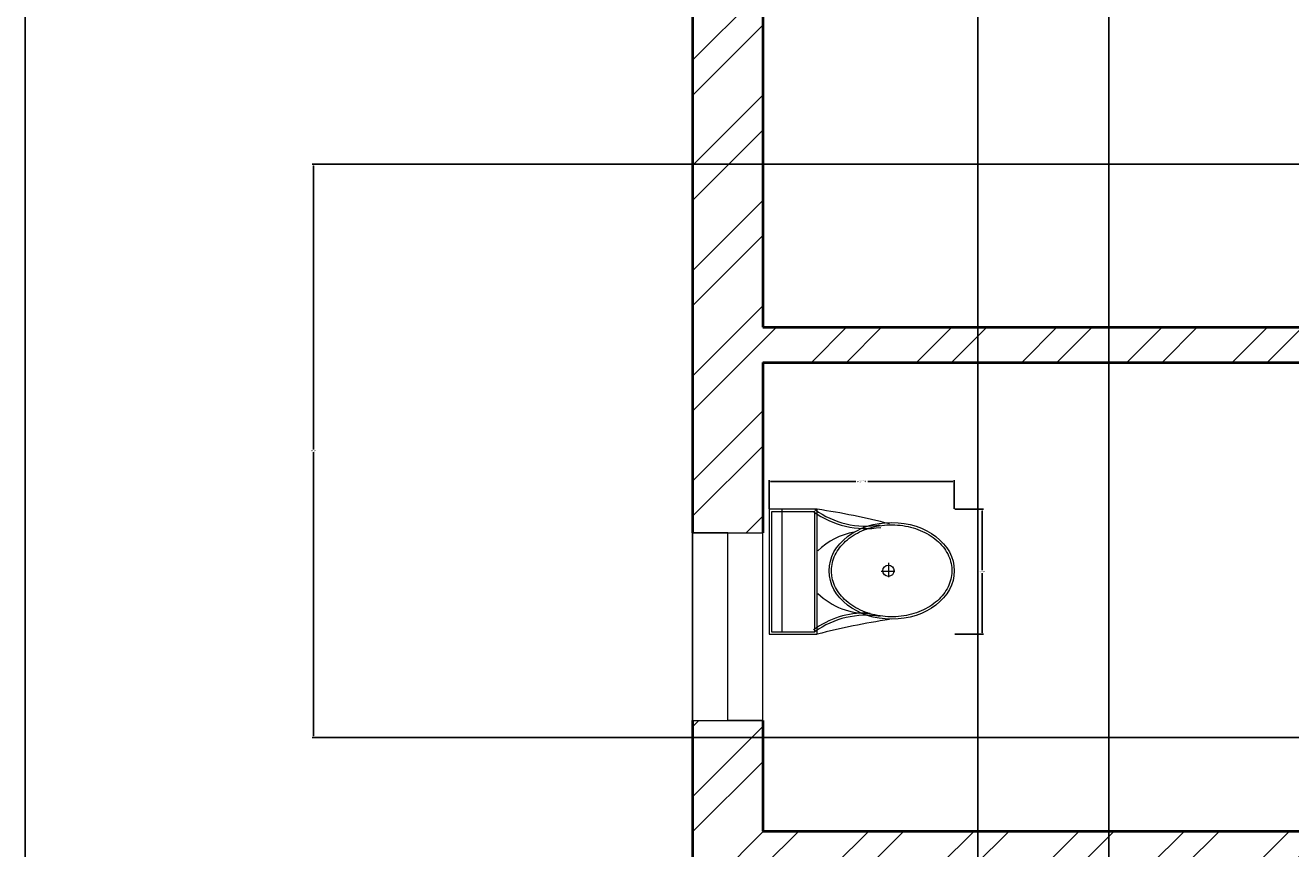
# Model space of a CAD drawing. Units: inches. Extents: x 1601 to 2297, y 1496 to 2631.
# Tile 35 of 57: x 1601 to 1763, y 2286 to 2391. Entities that reach past the tile are written whole.
import ezdxf

# ---------------------------------------------------------------- set-up
doc = ezdxf.new("R2010")
doc.units = ezdxf.units.IN
for name, color, linetype, lineweight in [('A-ANNO-DIMS', 2, 'Continuous', 18), ('A-ANNO-TTLB', 7, 'Continuous', 25), ('A-FLOR-FIXT', 9, 'Continuous', 20), ('A-GLAZ', 161, 'Continuous', 20), ('A-WALL', 7, 'Continuous', 40), ('A-WALL-PATT', 215, 'Continuous', 13)]:
    doc.layers.add(name, color=color, linetype=linetype, lineweight=lineweight)
doc.styles.get("Standard").update_dxf_attribs({"font": 'arial.ttf'})
doc.dimstyles.get("Standard").update_dxf_attribs({"dimtxt": 0.18, "dimasz": 0.18, "dimexe": 0.18, "dimexo": 0.0625, "dimgap": 0.09, "dimtad": 0, "dimtih": 1, "dimtoh": 1, "dimdec": 4, "dimzin": 0, "dimdsep": 46, "dimtxsty": 'Standard', "dimcen": 0.09, "dimadec": 0, "dimazin": 0, "dimtfac": 1, "dimtdec": 4, "dimtofl": 0, "dimtmove": 0, "dimatfit": 3, "dimfxl": 1, "dimtolj": 1, "dimtzin": 0, "dimarcsym": 0})

# ---------------------------------------------------------------- blocks, each defined once
blk = doc.blocks.new('A$C31115884')
for p, q in [((283.1, 497.7), (223.4, 497.7)), ((257.5, 466.4), (257.5, 523.2)), ((0, 200), (0, 0)), ((520, 200), (0, 200)), ((10, 190), (10, 10)), ((510, 190), (10, 190)), ((510, 10), (510, 190)), ((520, 0), (520, 200)), ((510, 54.5), (0, 54.5)), ((10, 10), (510, 10)), ((0, 0), (520, 0))]:
    blk.add_line(p, q)
blk.add_circle((255.6, 496.4), 23.6)
for centre, radius, start, end in [((2777.7, -204.6), 2807, 165.4549, 171.7133), ((3237, 905), 2807, 188.2867, 194.5451), ((-294.5, 403.3), 364.7, 324.2091, 9.3499), ((-294.5, 403.3), 374.7, 324.2091, 9.3499), ((805.8, 403.3), 364.7, 170.6501, 215.7909), ((139.5, 406.2), 293.5, 315.8436, 2.6563), ((805.8, 403.3), 374.7, 179.2036, 215.7909), ((383.6, 406.2), 293.5, 190.2774, 224.1564)]:
    blk.add_arc(centre, radius, start, end)
blk.add_ellipse((256.2, 509.9), major_axis=(0, -260.7), ratio=0.772727)
blk.add_open_spline([(256.2, 259.2), (263.1, 259.2), (270, 259.7), (287.8, 262.3), (298.7, 265.1), (319.9, 273.1), (330.2, 278.4), (350.1, 291.1), (359.7, 298.7), (377.7, 315.9), (386.2, 325.5), (401.7, 346.6), (408.8, 358.1), (421.3, 382.5), (426.8, 395.5), (435.9, 422.4), (439.5, 436.4), (444.8, 465.1), (446.5, 479.7), (447.9, 509.2), (447.6, 524), (445, 553.3), (442.7, 567.8), (436.3, 596), (432.1, 609.7), (421.9, 636), (416, 648.6), (402.5, 672.1), (395, 683), (378.6, 703), (369.8, 712.1), (351.1, 728), (341.3, 734.8), (320.9, 746.2), (310.4, 750.7), (288.9, 757.3), (278, 759.4), (256, 761), (245, 760.6), (223.1, 757.2), (212.3, 754.3), (191.1, 746.1), (180.8, 740.7), (160.9, 727.8), (151.4, 720.1), (133.5, 702.7), (125.1, 693), (109.6, 671.7), (102.6, 660.2), (90.2, 635.7), (84.9, 622.7), (76, 595.6), (72.4, 581.6), (67.2, 552.9), (65.6, 538.2), (64.4, 508.8), (64.8, 494), (67.5, 464.7), (69.9, 450.2), (76.6, 422), (80.8, 408.3), (91.1, 382.2), (97.2, 369.7), (110.8, 346.3), (118.4, 335.4), (134.8, 315.6), (143.7, 306.7), (162.4, 290.9), (172.3, 284.2), (192.8, 273), (203.3, 268.6), (224.8, 262.2), (235.8, 260.2), (249.9, 259.3), (253, 259.2), (256.2, 259.2)], degree=3, knots=[0, 0, 0, 0, 0.110105, 0.110105, 0.285049, 0.285049, 0.459994, 0.459994, 0.634938, 0.634938, 0.809882, 0.809882, 0.984827, 0.984827, 1.159771, 1.159771, 1.334715, 1.334715, 1.50966, 1.50966, 1.684604, 1.684604, 1.859549, 1.859549, 2.034493, 2.034493, 2.209437, 2.209437, 2.384382, 2.384382, 2.559326, 2.559326, 2.73427, 2.73427, 2.909215, 2.909215, 3.084159, 3.084159, 3.259103, 3.259103, 3.434048, 3.434048, 3.608992, 3.608992, 3.783936, 3.783936, 3.958881, 3.958881, 4.133825, 4.133825, 4.30877, 4.30877, 4.483714, 4.483714, 4.658658, 4.658658, 4.833603, 4.833603, 5.008547, 5.008547, 5.183491, 5.183491, 5.358436, 5.358436, 5.53338, 5.53338, 5.708324, 5.708324, 5.883269, 5.883269, 6.058213, 6.058213, 6.233158, 6.233158, 6.283185, 6.283185, 6.283185, 6.283185])
blk = doc.blocks.new('*D10')
at = {"layer": 'A-ANNO-DIMS', "color": 0, "lineweight": -2, "transparency": 16777216}
for p, q in [((1695.85, 2329.09), (1695.85, 2332.76)), ((1696.03, 2332.58), (1706.92, 2332.58)), ((1719.36, 2332.58), (1708.47, 2332.58)), ((1719.54, 2329.09), (1719.54, 2332.76))]:
    blk.add_line(p, q, dxfattribs=at)
at = {"layer": 'A-ANNO-DIMS', "color": 0, "transparency": 16777216}
for points in [[(1696.03, 2332.61), (1696.03, 2332.55), (1695.85, 2332.58)], [(1719.36, 2332.61), (1719.36, 2332.55), (1719.54, 2332.58)]]:
    blk.add_solid(points, dxfattribs=at)
at = {"layer": 'Defpoints', "color": 0, "transparency": 16777216}
for p in [(1719.54, 2332.58), (1695.85, 2329.02), (1719.54, 2329.02)]:
    blk.add_point(p, dxfattribs=at)
at = {"layer": 'A-ANNO-DIMS', "color": 0, "transparency": 16777216, "insert": (1707.69, 2332.58), "char_height": 0.18, "attachment_point": 5}
blk.add_mtext('\\A1;WC 24 TYP.', dxfattribs=at)
blk = doc.blocks.new('*D11')
at = {"layer": 'A-ANNO-DIMS', "color": 0, "lineweight": -2, "transparency": 16777216}
for p, q in [((1719.6, 2329.02), (1723.28, 2329.02)), ((1723.1, 2328.84), (1723.1, 2321.21)), ((1723.1, 2313.21), (1723.1, 2320.85)), ((1719.6, 2313.03), (1723.28, 2313.03))]:
    blk.add_line(p, q, dxfattribs=at)
at = {"layer": 'A-ANNO-DIMS', "color": 0, "transparency": 16777216}
for points in [[(1723.07, 2328.84), (1723.13, 2328.84), (1723.1, 2329.02)], [(1723.07, 2313.21), (1723.13, 2313.21), (1723.1, 2313.03)]]:
    blk.add_solid(points, dxfattribs=at)
at = {"layer": 'Defpoints', "color": 0, "transparency": 16777216}
for p in [(1719.54, 2329.02), (1719.54, 2313.03), (1723.1, 2313.03)]:
    blk.add_point(p, dxfattribs=at)
at = {"layer": 'A-ANNO-DIMS', "color": 0, "transparency": 16777216, "insert": (1723.1, 2321.03), "char_height": 0.18, "attachment_point": 5}
blk.add_mtext('\\A1;16 TYP.', dxfattribs=at)
blk = doc.blocks.new('*D32')
at = {"layer": 'A-ANNO-DIMS', "color": 0, "lineweight": -2, "transparency": 16777216}
for p, q in [((1686.04, 2031.39), (1686.04, 2581.06)), ((1686.22, 2580.88), (1703.91, 2580.88)), ((1722.39, 2580.88), (1704.7, 2580.88)), ((1722.57, 2031.39), (1722.57, 2581.06))]:
    blk.add_line(p, q, dxfattribs=at)
at = {"layer": 'A-ANNO-DIMS', "color": 0, "transparency": 16777216}
for points in [[(1686.22, 2580.91), (1686.22, 2580.85), (1686.04, 2580.88)], [(1722.39, 2580.91), (1722.39, 2580.85), (1722.57, 2580.88)]]:
    blk.add_solid(points, dxfattribs=at)
at = {"layer": 'Defpoints', "color": 0, "transparency": 16777216}
for p in [(1722.57, 2580.88), (1686.04, 2031.33), (1722.57, 2031.33)]:
    blk.add_point(p, dxfattribs=at)
at = {"layer": 'A-ANNO-DIMS', "color": 0, "transparency": 16777216, "insert": (1704.3, 2580.88), "char_height": 0.18, "attachment_point": 5}
blk.add_mtext('\\A1;36.53', dxfattribs=at)
blk = doc.blocks.new('*D36')
at = {"layer": 'A-ANNO-DIMS', "color": 0, "lineweight": -2, "transparency": 16777216}
for p, q in [((1686.04, 1635.39), (1686.04, 2581.06)), ((1686.22, 2580.88), (1712.36, 2580.88)), ((1739.15, 2580.88), (1713.01, 2580.88)), ((1739.33, 1635.39), (1739.33, 2581.06))]:
    blk.add_line(p, q, dxfattribs=at)
at = {"layer": 'A-ANNO-DIMS', "color": 0, "transparency": 16777216}
for points in [[(1686.22, 2580.91), (1686.22, 2580.85), (1686.04, 2580.88)], [(1739.15, 2580.91), (1739.15, 2580.85), (1739.33, 2580.88)]]:
    blk.add_solid(points, dxfattribs=at)
at = {"layer": 'Defpoints', "color": 0, "transparency": 16777216}
for p in [(1739.33, 2580.88), (1686.04, 1635.33), (1739.33, 1635.33)]:
    blk.add_point(p, dxfattribs=at)
at = {"layer": 'A-ANNO-DIMS', "color": 0, "transparency": 16777216, "insert": (1712.69, 2580.88), "char_height": 0.18, "attachment_point": 5}
blk.add_mtext('\\A1;53.3', dxfattribs=at)
blk = doc.blocks.new('*D48')
at = {"layer": 'A-ANNO-DIMS', "color": 0, "lineweight": -2, "transparency": 16777216}
for p, q in [((2030.97, 2373.19), (1637.31, 2373.19)), ((1637.49, 2373.01), (1637.49, 2336.69)), ((1637.49, 2300.01), (1637.49, 2336.33)), ((2030.97, 2299.83), (1637.31, 2299.83))]:
    blk.add_line(p, q, dxfattribs=at)
at = {"layer": 'A-ANNO-DIMS', "color": 0, "transparency": 16777216}
for points in [[(1637.46, 2373.01), (1637.52, 2373.01), (1637.49, 2373.19)], [(1637.46, 2300.01), (1637.52, 2300.01), (1637.49, 2299.83)]]:
    blk.add_solid(points, dxfattribs=at)
at = {"layer": 'Defpoints', "color": 0, "transparency": 16777216}
for p in [(1637.49, 2373.19), (2031.04, 2373.19), (2031.04, 2299.83)]:
    blk.add_point(p, dxfattribs=at)
at = {"layer": 'A-ANNO-DIMS', "color": 0, "transparency": 16777216, "insert": (1637.49, 2336.51), "char_height": 0.18, "attachment_point": 5}
blk.add_mtext('\\A1;73.37', dxfattribs=at)

msp = doc.modelspace()

# ---------------------------------------------------------------- hatches: boundary and pattern name
at = {"layer": 'A-WALL-PATT'}
h = msp.add_hatch(dxfattribs=at)
h.set_pattern_fill('ANSI32', color=256)
h.paths.add_polyline_path([(1842.0336, 2528.0767), (1842.0336, 2532.3254), (1686.0373, 2532.3254), (1686.0373, 2492.9493), (1695.0373, 2492.9493), (1695.0373, 2523.3254), (1827.0373, 2523.3254), (1827.0373, 2416.8254), (1834.6225, 2416.8254), (1834.6225, 2419.0754), (1834.6225, 2421.3254), (1831.5373, 2421.3254), (1831.5373, 2523.3254), (1842.0336, 2523.3254)])
h.paths.add_polyline_path([(1695.0373, 2432.9493), (1686.0373, 2432.9493), (1686.0373, 2325.989), (1695.0373, 2325.989), (1695.0373, 2347.8254), (1827.0373, 2347.8254), (1827.0373, 2287.8254), (1823.2991, 2287.8254), (1823.2991, 2283.3254), (1847.9422, 2283.3254), (1847.9422, 2285.5754), (1847.9422, 2287.8254), (1831.5373, 2287.8254), (1831.5373, 2347.8254), (1846.9946, 2347.8254), (1846.9946, 2350.0754), (1846.9946, 2352.3254), (1695.0373, 2352.3254)])
h.paths.add_polyline_path([(1807.1169, 1573.5395), (2055.0405, 1573.5395), (2055.0405, 1610.6322), (1807.1169, 1610.6322)], flags=9)
h.paths.add_polyline_path([(1841.1631, 1712.7967), (1870.3957, 1712.7967), (1870.3957, 1731.454), (1841.1631, 1731.454)], flags=9)
h.paths.add_polyline_path([(2144.3862, 1772.185), (2191.0233, 1772.185), (2191.0233, 1790.8423), (2144.3862, 1790.8423)], flags=9)
h.paths.add_polyline_path([(2143.0128, 1827.3312), (2177.9958, 1827.3312), (2177.9958, 1845.9886), (2143.0128, 1845.9886)], flags=9)
h.paths.add_polyline_path([(2041.2439, 1833.5691), (2070.8516, 1833.5691), (2070.8516, 1852.2264), (2041.2439, 1852.2264)], flags=9)
h.paths.add_polyline_path([(2097.2791, 1947.0598), (2134.2061, 1947.0598), (2134.2061, 1965.7171), (2097.2791, 1965.7171)], flags=9)
h.paths.add_polyline_path([(2214.995, 1904.3124), (2214.995, 1942.2899), (2196.3376, 1942.2899), (2196.3376, 1904.3124)], flags=9)
h.paths.add_polyline_path([(2186.6284, 2043.8031), (2219.7935, 2043.8031), (2219.7935, 2062.4605), (2186.6284, 2062.4605)], flags=9)
h.paths.add_polyline_path([(2064.0877, 2031.616), (2097.4949, 2031.616), (2097.4949, 2050.2734), (2064.0877, 2050.2734)], flags=9)
h.paths.add_polyline_path([(1973.1349, 1986.0688), (2008.4009, 1986.0688), (2008.4009, 2004.7261), (1973.1349, 2004.7261)], flags=9)
h.paths.add_polyline_path([(1976.3676, 2106.9635), (2005.7469, 2106.9635), (2005.7469, 2125.6209), (1976.3676, 2125.6209)], flags=9)
h.paths.add_polyline_path([(1991.7852, 2180.4863), (2027.0513, 2180.4863), (2027.0513, 2199.1437), (1991.7852, 2199.1437)], flags=9)
h.paths.add_polyline_path([(2106.1801, 2187.9359), (2152.2101, 2187.9359), (2152.2101, 2206.5932), (2106.1801, 2206.5932)], flags=9)
h.paths.add_polyline_path([(2148.6686, 2262.2542), (2182.318, 2262.2542), (2182.318, 2280.9115), (2148.6686, 2280.9115)], flags=9)
h.paths.add_polyline_path([(2041.6327, 2252.8147), (2071.2405, 2252.8147), (2071.2405, 2271.4721), (2041.6327, 2271.4721)], flags=9)
h.paths.add_polyline_path([(2063.9734, 2375.4265), (2100.9004, 2375.4265), (2100.9004, 2394.0839), (2063.9734, 2394.0839)], flags=9)
h.paths.add_polyline_path([(2216.4955, 2330.9748), (2216.4955, 2370.2654), (2197.8381, 2370.2654), (2197.8381, 2330.9748)], flags=9)
h.paths.add_polyline_path([(2179.1416, 2485.8687), (2212.3067, 2485.8687), (2212.3067, 2504.5261), (2179.1416, 2504.5261)], flags=9)
h.paths.add_polyline_path([(2078.7442, 2471.1516), (2112.1514, 2471.1516), (2112.1514, 2489.809), (2078.7442, 2489.809)], flags=9)
h.paths.add_polyline_path([(1915.9631, 2329.4668), (1952.8902, 2329.4668), (1952.8902, 2348.1241), (1915.9631, 2348.1241)], flags=9)
h.paths.add_polyline_path([(1904.3189, 2499.6709), (1940.4512, 2499.6709), (1940.4512, 2518.3282), (1904.3189, 2518.3282)], flags=9)
h.paths.add_polyline_path([(1892.3665, 2100.4595), (1925.6374, 2100.4595), (1925.6374, 2119.1169), (1892.3665, 2119.1169)], flags=9)
h.paths.add_polyline_path([(1909.2984, 1805.9631), (1946.2254, 1805.9631), (1946.2254, 1824.6205), (1909.2984, 1824.6205)], flags=9)
h.paths.add_polyline_path([(1934.6056, 1658.616), (1970.738, 1658.616), (1970.738, 1677.2733), (1934.6056, 1677.2733)], flags=9)
h.paths.add_polyline_path([(1711.2052, 1789.8902), (1750.0456, 1789.8902), (1750.0456, 1808.5476), (1711.2052, 1808.5476)], flags=9)
h.paths.add_polyline_path([(1742.7874, 1854.6743), (1771.9449, 1854.6743), (1771.9449, 1873.3317), (1742.7874, 1873.3317)], flags=9)
h.paths.add_polyline_path([(1807.3592, 1997.7912), (1850.1116, 1997.7912), (1850.1116, 2016.4486), (1807.3592, 2016.4486)], flags=9)
h.paths.add_polyline_path([(1717.4579, 2237.7844), (1760.2103, 2237.7844), (1760.2103, 2256.4417), (1717.4579, 2256.4417)], flags=9)
h.paths.add_polyline_path([(1780.9285, 2324.0623), (1810.086, 2324.0623), (1810.086, 2342.7197), (1780.9285, 2342.7197)], flags=25)
h.paths.add_polyline_path([(1837.696, 2449.2024), (1866.9286, 2449.2024), (1866.9286, 2467.8598), (1837.696, 2467.8598)], flags=9)
h.paths.add_polyline_path([(1712.7752, 2484.9404), (1751.6156, 2484.9404), (1751.6156, 2503.5977), (1712.7752, 2503.5977)], flags=25)
h = msp.add_hatch(dxfattribs=at)
h.set_pattern_fill('ANSI32', color=256)
h.paths.add_polyline_path([(1695.0373, 2283.3254), (1801.5627, 2283.3254), (1801.5627, 2285.5754), (1801.5627, 2287.8254), (1695.0373, 2287.8254), (1695.0373, 2301.989), (1690.5373, 2301.989), (1686.0373, 2301.989), (1686.0373, 2233.8724), (1695.0373, 2233.8724)])

# ---------------------------------------------------------------- linework, layer by layer
at = {"layer": 'A-ANNO-TTLB'}
msp.add_lwpolyline([(1600.5933, 2631.1477), (2297.129, 2631.1477), (2297.129, 1496.1026), (1600.5933, 1496.1026)], close=True, dxfattribs=at)
at = {"layer": 'A-GLAZ'}
for p, q in [((1690.5373, 2325.989), (1686.0373, 2325.989)), ((1686.0373, 2325.989), (1695.0373, 2325.989)), ((1686.0373, 2325.989), (1686.0373, 2302.7018)), ((1690.5373, 2301.989), (1690.5373, 2325.989)), ((1695.0373, 2301.989), (1695.0373, 2325.989)), ((1686.0373, 2302.7018), (1686.0373, 2301.989)), ((1686.0373, 2301.989), (1695.0373, 2301.989)), ((1695.0373, 2301.989), (1690.5373, 2301.989))]:
    msp.add_line(p, q, dxfattribs=at)
at = {"layer": 'A-WALL'}
for p, q in [((1686.0373, 2432.9493), (1686.0373, 2325.989)), ((1695.0373, 2432.9493), (1695.0373, 2352.3254)), ((1695.0373, 2352.3254), (1848.92, 2352.3254)), ((1695.0373, 2347.8254), (1827.0373, 2347.8254)), ((1695.0373, 2347.8254), (1695.0373, 2325.989)), ((1686.0373, 2301.989), (1686.0373, 2233.8724)), ((1695.0373, 2301.989), (1695.0373, 2287.8254)), ((1695.0373, 2287.8254), (1803.0227, 2287.8254))]:
    msp.add_line(p, q, dxfattribs=at)

# ---------------------------------------------------------------- block references
at = {"layer": 'A-FLOR-FIXT', "xscale": 0.0307498789965588, "yscale": 0.0307498789965588, "zscale": 0.0307498789965588, "rotation": 270}
msp.add_blockref('A$C31115884', (1695.8474, 2329.0246), dxfattribs=at)

# ---------------------------------------------------------------- dimensions: what is measured, and where the dimension line sits
at = {"layer": 'A-ANNO-DIMS'}
for base, p1, p2, override, picture, middle in [((1722.5687, 2580.8754), (1686.0373, 2031.3254), (1722.5687, 2031.3254), {"dimdec": 2, "dimlfac": 1, "dimrnd": 0, "dimzin": 0, "dimdsep": 46, "dimlunit": 2}, '*D32', (1704.303, 2580.8754)), ((1739.3335, 2580.8754), (1686.0373, 1635.3254), (1739.3335, 1635.3254), {"dimdec": 1, "dimlfac": 1, "dimrnd": 0, "dimzin": 0, "dimdsep": 46, "dimlunit": 2}, '*D36', (1712.6854, 2580.8754))]:
    dim = msp.add_linear_dim(base=base, p1=p1, p2=p2, dimstyle='Standard', override=override, dxfattribs=at)
    dim.commit()
    dim.dimension.update_dxf_attribs({"geometry": picture, "text_midpoint": middle})
dim = msp.add_linear_dim(base=(1637.4873, 2373.1914), p1=(2031.0373, 2299.8254), p2=(2031.0373, 2373.1914), angle=90, dimstyle='Standard', override={"dimdec": 2, "dimlfac": 1, "dimrnd": 0, "dimzin": 0, "dimdsep": 46, "dimlunit": 2}, dxfattribs=at)
dim.commit()
dim.dimension.update_dxf_attribs({"geometry": '*D48', "text_midpoint": (1637.4873, 2336.5084)})
dim = msp.add_linear_dim(base=(1719.5423, 2332.5788), p1=(1695.8474, 2329.0246), p2=(1719.5423, 2329.0246), text='WC <> TYP.', dimstyle='Standard', override={"dimdec": 0, "dimlfac": 1, "dimrnd": 0, "dimzin": 0, "dimdsep": 46, "dimlunit": 2}, dxfattribs=at)
dim.commit()
dim.dimension.update_dxf_attribs({"geometry": '*D10', "text_midpoint": (1707.6949, 2332.5788)})
dim = msp.add_linear_dim(base=(1723.0966, 2313.0346), p1=(1719.5423, 2329.0246), p2=(1719.5423, 2313.0346), angle=270, text='<> TYP.', dimstyle='Standard', override={"dimdec": 0, "dimlfac": 1, "dimrnd": 0, "dimzin": 0, "dimdsep": 46, "dimlunit": 2}, dxfattribs=at)
dim.commit()
dim.dimension.update_dxf_attribs({"geometry": '*D11', "text_midpoint": (1723.0966, 2321.0296)})

doc.saveas('drawing.dxf')
